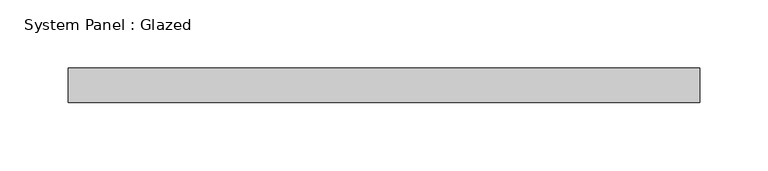
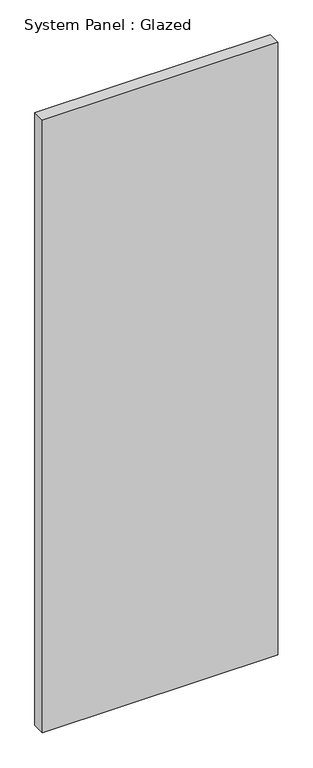
"""IFC4 building model written with IfcOpenShell, lengths in millimetres: plate geometry, System Panel : Glazed."""

from ifc_helpers import new_model, si_unit, origin, origin_with_axes, place, context, project, spatial, polyline, outline, extrude, source, transform, mapped, element, save


def system_panel_glazed_14b3f2be(model_context):
    return source(origin(), model_context, "Body", "SweptSolid", [
        extrude(outline(polyline([(231.775, 19.05), (-231.775, 19.05), (-231.775, 44.45), (231.775, 44.45), (231.775, 19.05)])), origin_with_axes(), (0.0, 0.0, 1.0), 1274.8499484),
    ])


if __name__ == "__main__":
    model = new_model("IFC4")
    model_context = context("Model", 3, world=origin())
    ifc_project = project(units=[si_unit("LENGTHUNIT", "METRE", prefix="MILLI")], contexts=[model_context])
    site = spatial("IfcSite", under=ifc_project)
    building = spatial("IfcBuilding", under=site)
    placement = place(None, origin())
    system_panel_glazed_shape = system_panel_glazed_14b3f2be(model_context)
    element("IfcPlate", 1, ObjectType="System Panel : Glazed", at=placement, inside=building, context=model_context, shape_type="MappedRepresentation", body=[
        mapped(system_panel_glazed_shape, transform((0.0, 0.0, 0.0), x_axis=(1.0, 0.0, 0.0), y_axis=(0.0, 1.0, 0.0), z_axis=(0.0, 0.0, 1.0))),
    ])
    save(model, "model.ifc")

# Revit data of these elements
# Type "System Panel : Glazed"
#   Construction Type Id = "GSP4R"
#   Analytic Construction = "1/8 in Pilkington single glazing"
#   Visual Light Transmittance = 0.9
#   Solar Heat Gain Coefficient = 0.86
#   Heat Transfer Coefficient (U) = 1.18115 BTU/(h·ft²·°F)
#   Define Thermal Properties by = 1
# Element 1 (IfcPlate, "System Panel : Glazed")
#   Materials on its faces: "Glass"
# Materials
#   "Glass": class "Glass", colour RGB 0 128 192, transparency 0.75, Description = "Soda Lime Glass", Cost = 0
